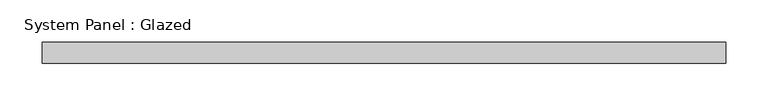
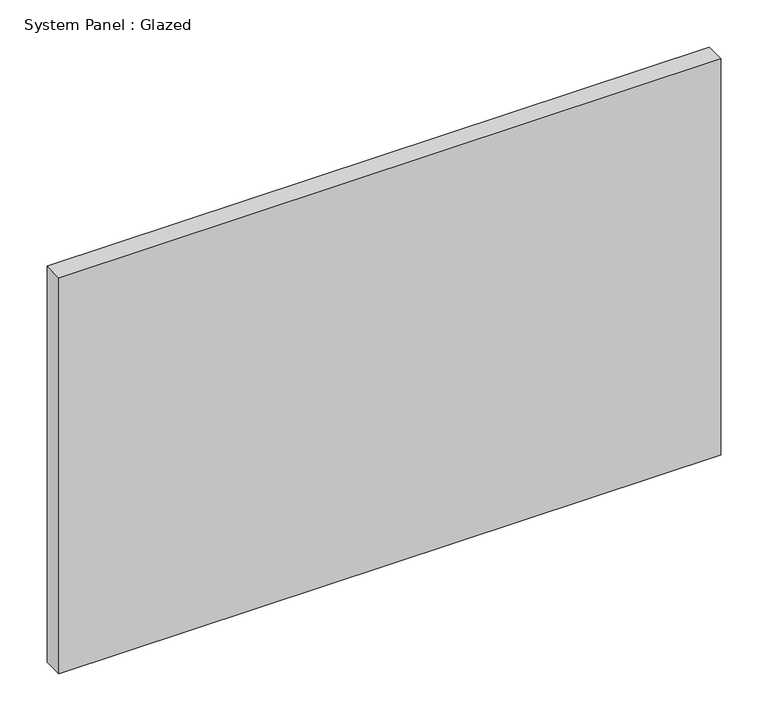
"""IFC4 building model written with IfcOpenShell, lengths in millimetres: plate geometry, System Panel : Glazed."""

from ifc_helpers import new_model, si_unit, origin, origin_with_axes, place, context, project, spatial, polyline, outline, extrude, source, transform, mapped, element, save


def system_panel_glazed_9a27d744(model_context):
    return source(origin(), model_context, "Body", "SweptSolid", [
        extrude(outline(polyline([(406.4, 19.05), (-406.4, 19.05), (-406.4, 44.45), (406.4, 44.45), (406.4, 19.05)])), origin_with_axes(), (0.0, 0.0, 1.0), 514.35),
    ])


if __name__ == "__main__":
    model = new_model("IFC4")
    model_context = context("Model", 3, world=origin())
    ifc_project = project(units=[si_unit("LENGTHUNIT", "METRE", prefix="MILLI")], contexts=[model_context])
    site = spatial("IfcSite", under=ifc_project)
    building = spatial("IfcBuilding", under=site)
    placement = place(None, origin())
    system_panel_glazed_shape = system_panel_glazed_9a27d744(model_context)
    element("IfcPlate", 1, ObjectType="System Panel : Glazed", at=placement, inside=building, context=model_context, shape_type="MappedRepresentation", body=[
        mapped(system_panel_glazed_shape, transform((0.0, 0.0, 0.0), x_axis=(1.0, 0.0, 0.0), y_axis=(0.0, 1.0, 0.0), z_axis=(0.0, 0.0, 1.0))),
    ])
    save(model, "model.ifc")

# Revit data of these elements
# Type "System Panel : Glazed"
#   Construction Type Id = "GSP4R"
#   Analytic Construction = "1/8 in Pilkington single glazing"
#   Visual Light Transmittance = 0.9
#   Solar Heat Gain Coefficient = 0.86
#   Heat Transfer Coefficient (U) = 1.18115 BTU/(h·ft²·°F)
#   Define Thermal Properties by = 1
# Element 1 (IfcPlate, "System Panel : Glazed")
#   Materials on its faces: "Glass"
# Materials
#   "Glass": class "Glass", colour RGB 0 128 192, transparency 0.75, Description = "Soda Lime Glass", Cost = 0
